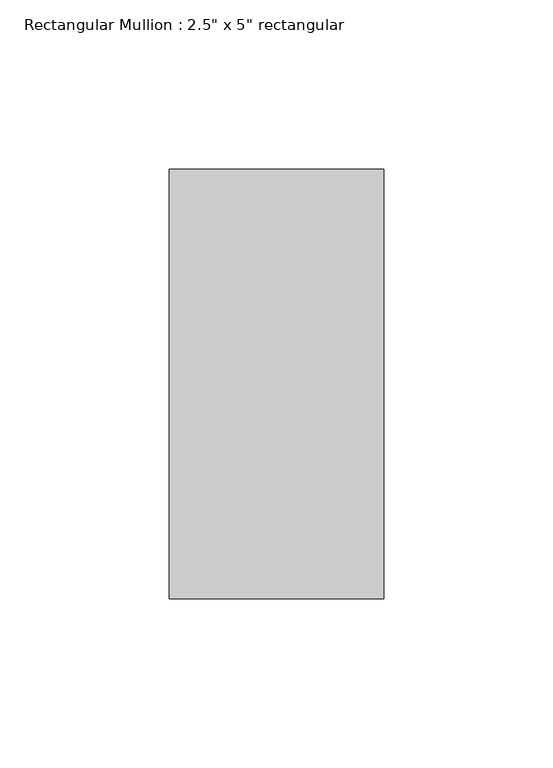
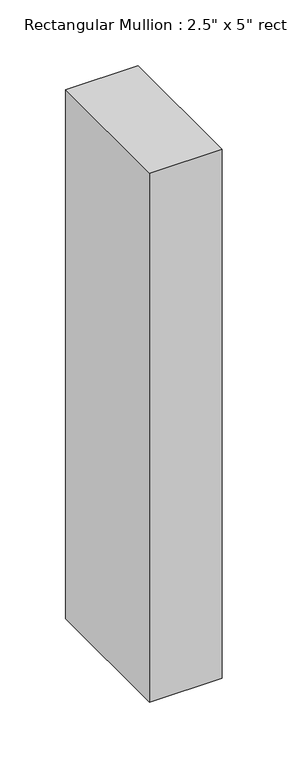
"""IFC4 building model written with IfcOpenShell, lengths in millimetres: member geometry."""

from ifc_helpers import new_model, si_unit, frame, origin, place, context, project, spatial, polyline, outline, extrude, source, transform, mapped, element, save


def member_285d49a4(model_context):
    return source(origin(), model_context, "Body", "SweptSolid", [
        extrude(outline(polyline([(0.0, 63.5), (0.0, -63.5), (-63.5, -63.5), (-63.5, 63.5), (0.0, 63.5)])), frame((0.0, 0.0, -489.8381005), z_axis=(0.0, 0.0, 1.0), x_axis=(1.0, 0.0, 0.0)), (0.0, 0.0, 1.0), 489.8381005),
    ])


if __name__ == "__main__":
    model = new_model("IFC4")
    model_context = context("Model", 3, world=origin())
    ifc_project = project(units=[si_unit("LENGTHUNIT", "METRE", prefix="MILLI")], contexts=[model_context])
    site = spatial("IfcSite", under=ifc_project)
    building = spatial("IfcBuilding", under=site)
    placement = place(None, origin())
    member_shape = member_285d49a4(model_context)
    element("IfcMember", 1, ObjectType="Rectangular Mullion : 2.5\" x 5\" rectangular", at=placement, inside=building, context=model_context, shape_type="MappedRepresentation", body=[
        mapped(member_shape, transform((0.0, 0.0, 0.0), x_axis=(1.0, 0.0, 0.0), y_axis=(0.0, 1.0, 0.0), z_axis=(0.0, 0.0, 1.0))),
    ])
    save(model, "model.ifc")

# Revit data of these elements
# Type "Rectangular Mullion : 2.5\" x 5\" rectangular"
#   built-in parameter 1007304 = 0.416667 (stored number, unit not read)
#   built-in parameter 1007301 = 0.104167 (stored number, unit not read)
#   built-in parameter 1007300 = 0.104167 (stored number, unit not read)
# Element 1 (IfcMember, "Rectangular Mullion : 2.5\" x 5\" rectangular")
#   Materials on its faces: "Aluminum"
# Materials
#   "Aluminum": class "Metal", colour RGB 247 247 247, transparency 0, Description = "Aluminum 6061", Cost = 0
